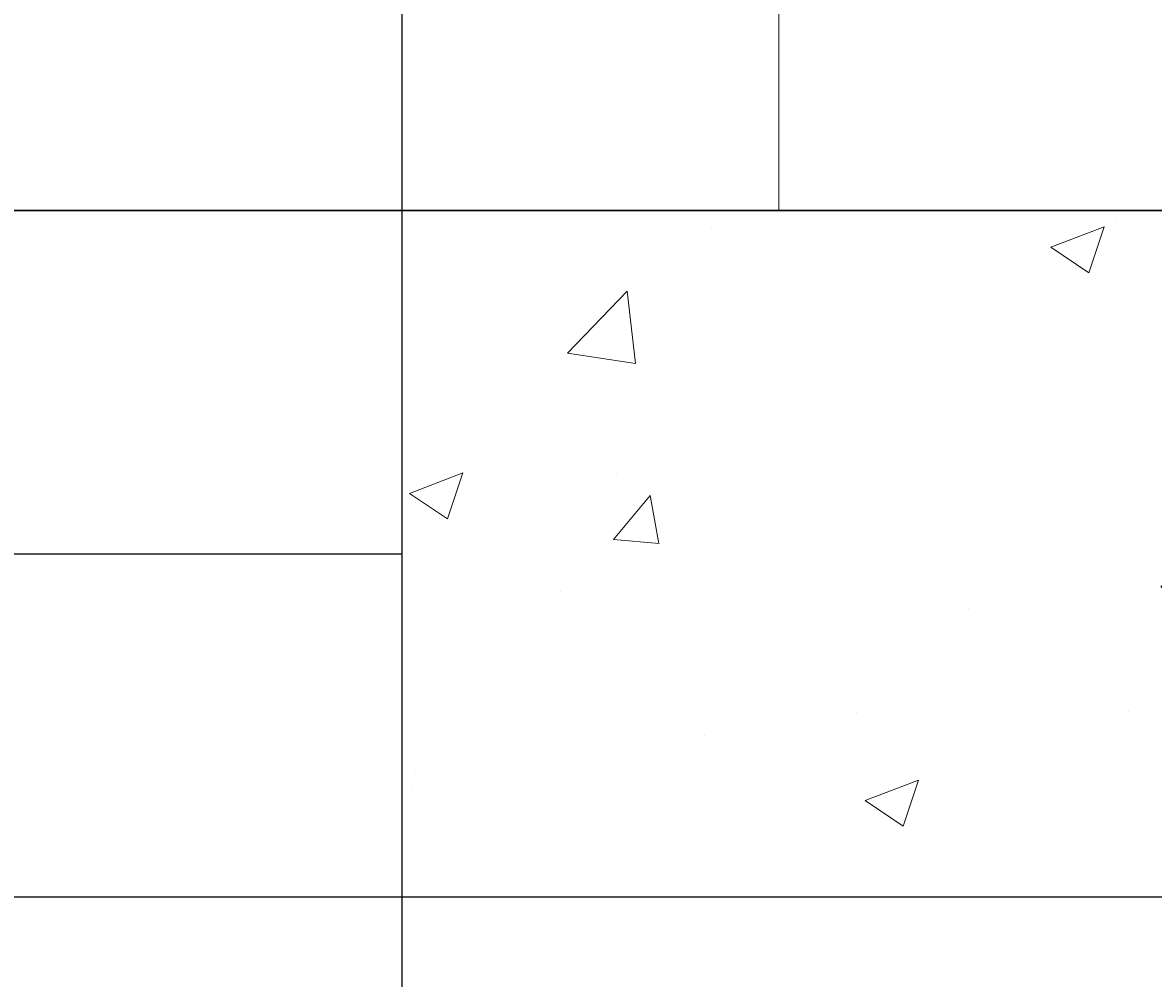
# Model space of a CAD drawing. Units: inches. Extents: x 37 to 824, y -700 to 234.
# Tile 14 of 77: x 348 to 378, y -606 to -581. Entities that reach past the tile are written whole.
import ezdxf

# ---------------------------------------------------------------- set-up
doc = ezdxf.new("R2010")
doc.units = ezdxf.units.IN
doc.header["$MEASUREMENT"] = 0
for name, color, linetype, lineweight in [('A-ANNO-DIMS', 2, 'Continuous', 18), ('A-ELEV', 3, 'Continuous', 25), ('A-ELEV-PATT', 8, 'Continuous', 13)]:
    doc.layers.add(name, color=color, linetype=linetype, lineweight=lineweight)
doc.styles.get("Standard").update_dxf_attribs({"font": 'arial.ttf'})
doc.dimstyles.get("Standard").update_dxf_attribs({"dimtxt": 0.18, "dimasz": 0.18, "dimexe": 0.18, "dimexo": 0.0625, "dimgap": 0.09, "dimtad": 0, "dimtih": 1, "dimtoh": 1, "dimdec": 1, "dimzin": 0, "dimdsep": 46, "dimlunit": 4, "dimtxsty": 'Standard', "dimcen": 0.09, "dimadec": 0, "dimazin": 0, "dimtfac": 1, "dimtdec": 1, "dimtofl": 0, "dimtmove": 0, "dimatfit": 3, "dimfxl": 1, "dimtolj": 1, "dimtzin": 0, "dimarcsym": 0})

# ---------------------------------------------------------------- blocks, each defined once
blk = doc.blocks.new('*D28')
at = {"layer": 'A-ANNO-DIMS', "color": 0, "lineweight": -2, "ltscale": 0.5, "transparency": 16777216}
for p, q in [((255.14, -537.627), (449.868, -537.627)), ((449.688, -543.627), (449.688, -558.537)), ((449.688, -579.627), (449.688, -564.717)), ((294.64, -585.627), (449.868, -585.627))]:
    blk.add_line(p, q, dxfattribs=at)
at = {"layer": 'A-ANNO-DIMS', "color": 0, "ltscale": 0.5, "transparency": 16777216}
for points in [[(448.688, -543.627), (450.688, -543.627), (449.688, -537.627)], [(448.688, -579.627), (450.688, -579.627), (449.688, -585.627)]]:
    blk.add_solid(points, dxfattribs=at)
at = {"layer": 'Defpoints', "color": 0, "ltscale": 0.5, "transparency": 16777216}
for p in [(255.077, -537.627), (294.577, -585.627), (449.688, -585.627)]:
    blk.add_point(p, dxfattribs=at)
at = {"layer": 'A-ANNO-DIMS', "color": 0, "ltscale": 0.5, "transparency": 16777216, "insert": (449.688, -561.627), "char_height": 6, "attachment_point": 5}
blk.add_mtext("\\A1;4'", dxfattribs=at)
blk = doc.blocks.new('*D70')
at = {"layer": 'A-ANNO-DIMS', "color": 0, "lineweight": -2, "ltscale": 0.5, "transparency": 16777216}
for p, q in [((299.077, -585.69), (299.077, -699.594)), ((358.132, -585.69), (358.132, -699.594)), ((299.257, -699.414), (328.202, -699.414)), ((357.952, -699.414), (329.008, -699.414))]:
    blk.add_line(p, q, dxfattribs=at)
at = {"layer": 'A-ANNO-DIMS', "color": 0, "ltscale": 0.5, "transparency": 16777216}
for points in [[(299.257, -699.384), (299.257, -699.444), (299.077, -699.414)], [(357.952, -699.384), (357.952, -699.444), (358.132, -699.414)]]:
    blk.add_solid(points, dxfattribs=at)
at = {"layer": 'Defpoints', "color": 0, "ltscale": 0.5, "transparency": 16777216}
for p in [(299.077, -585.627), (358.132, -585.627), (358.132, -699.414)]:
    blk.add_point(p, dxfattribs=at)
at = {"layer": 'A-ANNO-DIMS', "color": 0, "ltscale": 0.5, "transparency": 16777216, "insert": (328.605, -699.414), "char_height": 0.18, "attachment_point": 5}
blk.add_mtext('\\A1;4\'-11"', dxfattribs=at)
blk = doc.blocks.new('*D71')
at = {"layer": 'A-ANNO-DIMS', "color": 0, "lineweight": -2, "ltscale": 0.5, "transparency": 16777216}
for p, q in [((358.132, -585.69), (358.132, -699.594)), ((428.077, -585.69), (428.077, -699.594)), ((358.312, -699.414), (392.706, -699.414)), ((427.897, -699.414), (393.504, -699.414))]:
    blk.add_line(p, q, dxfattribs=at)
at = {"layer": 'A-ANNO-DIMS', "color": 0, "ltscale": 0.5, "transparency": 16777216}
for points in [[(358.312, -699.384), (358.312, -699.444), (358.132, -699.414)], [(427.897, -699.384), (427.897, -699.444), (428.077, -699.414)]]:
    blk.add_solid(points, dxfattribs=at)
at = {"layer": 'Defpoints', "color": 0, "ltscale": 0.5, "transparency": 16777216}
for p in [(358.132, -585.627), (428.077, -585.627), (428.077, -699.414)]:
    blk.add_point(p, dxfattribs=at)
at = {"layer": 'A-ANNO-DIMS', "color": 0, "ltscale": 0.5, "transparency": 16777216, "insert": (393.105, -699.414), "char_height": 0.18, "attachment_point": 5}
blk.add_mtext('\\A1;5\'-10"', dxfattribs=at)

msp = doc.modelspace()

# ---------------------------------------------------------------- hatches: boundary and pattern name
at = {"layer": 'A-ELEV-PATT', "ltscale": 0.5}
h = msp.add_hatch(dxfattribs=at)
h.set_pattern_fill('AR-BRSTD', color=256, scale=4)
h.paths.add_polyline_path([(299.077, -489.627), (358.132, -489.627), (358.132, -585.627), (428.077, -585.627), (428.077, -465.627), (161.077, -465.627), (161.077, -585.627), (299.077, -585.627)])
h.paths.add_polyline_path([(205.077, -537.627), (205.077, -489.627), (255.077, -489.627), (255.077, -537.627)], flags=16)
h = msp.add_hatch(dxfattribs=at)
h.set_pattern_fill('AR-CONC', color=256, scale=2)
h.paths.add_polyline_path([(299.077, -585.627), (161.077, -585.627), (161.077, -603.627), (299.077, -603.627)])
h.paths.add_polyline_path([(428.077, -585.627), (358.132, -585.627), (358.132, -603.627), (428.077, -603.627)])

# ---------------------------------------------------------------- linework, layer by layer
at = {"layer": 'A-ELEV', "ltscale": 0.5}
for p, q in [((299.077, -585.627), (358.132, -585.627)), ((358.132, -585.627), (358.132, -603.627)), ((299.077, -594.627), (358.132, -594.627))]:
    msp.add_line(p, q, dxfattribs=at)
for points in [[(161.077, -465.627), (428.077, -465.627), (428.077, -585.627), (161.077, -585.627)], [(299.077, -489.627), (358.132, -489.627), (358.132, -585.627), (299.077, -585.627)], [(161.077, -585.627), (428.077, -585.627), (428.077, -603.627), (161.077, -603.627)]]:
    msp.add_lwpolyline(points, close=True, dxfattribs=at)

# ---------------------------------------------------------------- dimensions: what is measured, and where the dimension line sits
at = {"layer": 'A-ANNO-DIMS', "ltscale": 0.5}
dim = msp.add_linear_dim(base=(449.688, -585.627), p1=(255.077, -537.627), p2=(294.577, -585.627), angle=90, dimstyle='Standard', override={"dimtxt": 6, "dimasz": 6, "dimclrd": 0, "dimclre": 0, "dimclrt": 0}, dxfattribs=at)
dim.commit()
dim.dimension.update_dxf_attribs({"geometry": '*D28', "text_midpoint": (449.688, -561.627)})
for base, p1, p2, picture, middle in [((358.132, -699.414), (299.077, -585.627), (358.132, -585.627), '*D70', (328.605, -699.414)), ((428.077, -699.414), (358.132, -585.627), (428.077, -585.627), '*D71', (393.105, -699.414))]:
    dim = msp.add_linear_dim(base=base, p1=p1, p2=p2, dimstyle='Standard', override={"dimdec": 1, "dimlfac": 1, "dimrnd": 0, "dimzin": 1, "dimdsep": 46, "dimlunit": 4, "dimfrac": 2}, dxfattribs=at)
    dim.commit()
    dim.dimension.update_dxf_attribs({"geometry": picture, "text_midpoint": middle})

doc.saveas('drawing.dxf')
